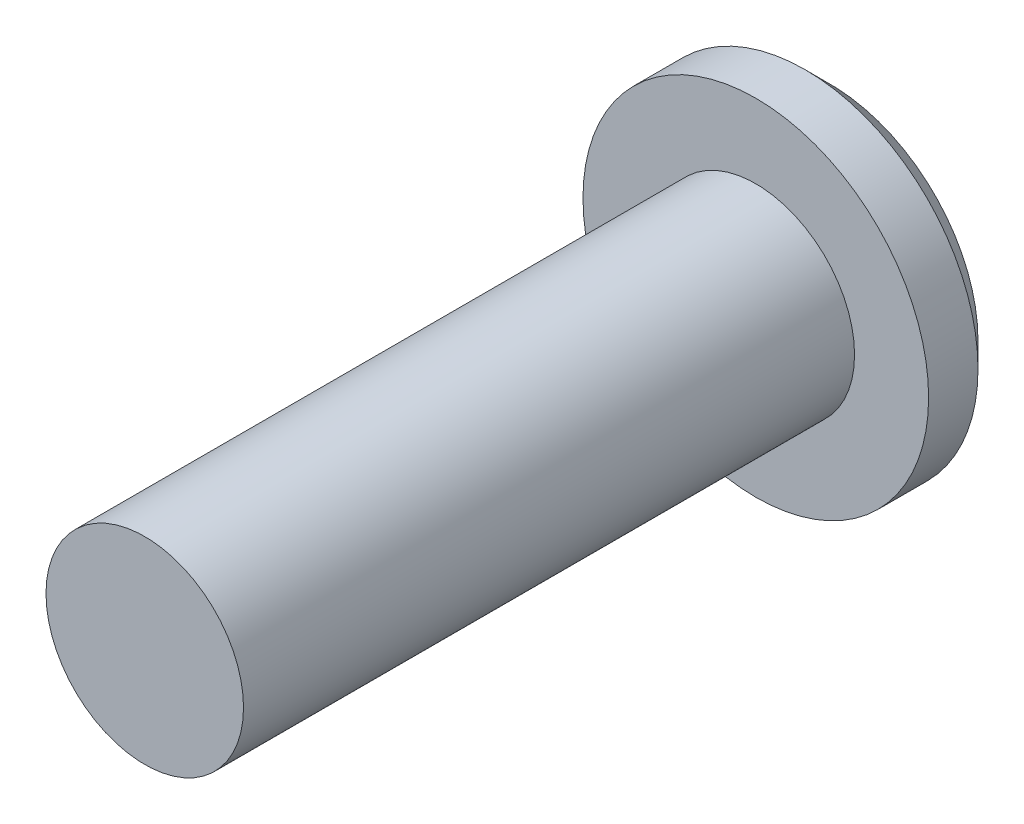
ISO-10303-21;
HEADER;
FILE_DESCRIPTION(('STEP AP214'),'2;1');
FILE_NAME('part.step','',(''),(''),'','','');
FILE_SCHEMA(('AUTOMOTIVE_DESIGN { 1 0 10303 214 1 1 1 1 }'));
ENDSEC;
DATA;
#1=APPLICATION_CONTEXT('core data for automotive mechanical design processes');
#2=APPLICATION_PROTOCOL_DEFINITION('international standard','automotive_design',2000,#1);
#3=PRODUCT_CONTEXT('',#1,'mechanical');
#4=PRODUCT('Part','Part','',(#3));
#5=PRODUCT_RELATED_PRODUCT_CATEGORY('part','',(#4));
#6=PRODUCT_DEFINITION_FORMATION('','',#4);
#7=PRODUCT_DEFINITION_CONTEXT('part definition',#1,'design');
#8=PRODUCT_DEFINITION('design','',#6,#7);
#9=PRODUCT_DEFINITION_SHAPE('','',#8);
#10=(LENGTH_UNIT() NAMED_UNIT(*) SI_UNIT(.MILLI.,.METRE.));
#11=(NAMED_UNIT(*) PLANE_ANGLE_UNIT() SI_UNIT($,.RADIAN.));
#12=(NAMED_UNIT(*) SI_UNIT($,.STERADIAN.) SOLID_ANGLE_UNIT());
#13=UNCERTAINTY_MEASURE_WITH_UNIT(LENGTH_MEASURE(1.E-05),#10,'distance_accuracy_value','');
#14=(GEOMETRIC_REPRESENTATION_CONTEXT(3) GLOBAL_UNCERTAINTY_ASSIGNED_CONTEXT((#13)) GLOBAL_UNIT_ASSIGNED_CONTEXT((#10,
#11,#12)) REPRESENTATION_CONTEXT('',''));
#15=CARTESIAN_POINT('',(0.,0.,0.));
#16=DIRECTION('',(0.,0.,1.));
#17=DIRECTION('',(1.,0.,0.));
#18=AXIS2_PLACEMENT_3D('',#15,#16,#17);
#19=CARTESIAN_POINT('',(0.,0.,3.));
#20=DIRECTION('',(0.,0.,-1.));
#21=DIRECTION('',(-1.,0.,0.));
#22=AXIS2_PLACEMENT_3D('',#19,#20,#21);
#23=CYLINDRICAL_SURFACE('',#22,7.);
#24=CARTESIAN_POINT('',(0.,0.,0.999999999999999));
#25=DIRECTION('',(0.,0.,1.));
#26=DIRECTION('',(1.,0.,0.));
#27=AXIS2_PLACEMENT_3D('',#24,#25,#26);
#28=CIRCLE('',#27,7.);
#29=CARTESIAN_POINT('',(7.,0.,0.999999999999999));
#30=VERTEX_POINT('',#29);
#31=EDGE_CURVE('E52',#30,#30,#28,.T.);
#32=ORIENTED_EDGE('',*,*,#31,.T.);
#33=EDGE_LOOP('',(#32));
#34=FACE_BOUND('',#33,.T.);
#35=CARTESIAN_POINT('',(0.,0.,3.));
#36=DIRECTION('',(0.,0.,1.));
#37=DIRECTION('',(1.,0.,0.));
#38=AXIS2_PLACEMENT_3D('',#35,#36,#37);
#39=CIRCLE('',#38,7.);
#40=CARTESIAN_POINT('',(7.,0.,3.));
#41=VERTEX_POINT('',#40);
#42=EDGE_CURVE('E61',#41,#41,#39,.T.);
#43=ORIENTED_EDGE('',*,*,#42,.F.);
#44=EDGE_LOOP('',(#43));
#45=FACE_BOUND('',#44,.T.);
#46=ADVANCED_FACE('F44',(#34,#45),#23,.T.);
#47=CARTESIAN_POINT('',(0.,0.,3.));
#48=DIRECTION('',(0.,0.,1.));
#49=DIRECTION('',(1.,0.,0.));
#50=AXIS2_PLACEMENT_3D('',#47,#48,#49);
#51=PLANE('',#50);
#52=CARTESIAN_POINT('',(0.,0.,3.));
#53=DIRECTION('',(0.,0.,1.));
#54=DIRECTION('',(1.,0.,0.));
#55=AXIS2_PLACEMENT_3D('',#52,#53,#54);
#56=CIRCLE('',#55,4.);
#57=CARTESIAN_POINT('',(4.,0.,3.));
#58=VERTEX_POINT('',#57);
#59=EDGE_CURVE('E60',#58,#58,#56,.T.);
#60=ORIENTED_EDGE('',*,*,#59,.F.);
#61=EDGE_LOOP('',(#60));
#62=FACE_BOUND('',#61,.T.);
#63=ORIENTED_EDGE('',*,*,#42,.T.);
#64=EDGE_LOOP('',(#63));
#65=FACE_BOUND('',#64,.T.);
#66=ADVANCED_FACE('F78',(#62,#65),#51,.T.);
#67=CARTESIAN_POINT('',(0.,0.,0.));
#68=DIRECTION('',(0.,0.,1.));
#69=DIRECTION('',(1.,0.,0.));
#70=AXIS2_PLACEMENT_3D('',#67,#68,#69);
#71=PLANE('',#70);
#72=CARTESIAN_POINT('',(0.,0.,0.));
#73=DIRECTION('',(0.,0.,1.));
#74=DIRECTION('',(1.,0.,0.));
#75=AXIS2_PLACEMENT_3D('',#72,#73,#74);
#76=CIRCLE('',#75,6.);
#77=CARTESIAN_POINT('',(6.,0.,0.));
#78=VERTEX_POINT('',#77);
#79=EDGE_CURVE('E10',#78,#78,#76,.F.);
#80=ORIENTED_EDGE('',*,*,#79,.T.);
#81=EDGE_LOOP('',(#80));
#82=FACE_BOUND('',#81,.T.);
#83=ADVANCED_FACE('F73',(#82),#71,.F.);
#84=CARTESIAN_POINT('',(0.,0.,27.75));
#85=DIRECTION('',(0.,0.,-1.));
#86=DIRECTION('',(-1.,0.,0.));
#87=AXIS2_PLACEMENT_3D('',#84,#85,#86);
#88=CYLINDRICAL_SURFACE('',#87,4.);
#89=CARTESIAN_POINT('',(0.,0.,27.75));
#90=DIRECTION('',(0.,0.,1.));
#91=DIRECTION('',(1.,0.,0.));
#92=AXIS2_PLACEMENT_3D('',#89,#90,#91);
#93=CIRCLE('',#92,4.);
#94=CARTESIAN_POINT('',(4.,0.,27.75));
#95=VERTEX_POINT('',#94);
#96=EDGE_CURVE('E64',#95,#95,#93,.T.);
#97=ORIENTED_EDGE('',*,*,#96,.F.);
#98=EDGE_LOOP('',(#97));
#99=FACE_BOUND('',#98,.T.);
#100=ORIENTED_EDGE('',*,*,#59,.T.);
#101=EDGE_LOOP('',(#100));
#102=FACE_BOUND('',#101,.T.);
#103=ADVANCED_FACE('F75',(#99,#102),#88,.T.);
#104=CARTESIAN_POINT('',(0.,0.,27.75));
#105=DIRECTION('',(0.,0.,1.));
#106=DIRECTION('',(1.,0.,0.));
#107=AXIS2_PLACEMENT_3D('',#104,#105,#106);
#108=PLANE('',#107);
#109=ORIENTED_EDGE('',*,*,#96,.T.);
#110=EDGE_LOOP('',(#109));
#111=FACE_BOUND('',#110,.T.);
#112=ADVANCED_FACE('F67',(#111),#108,.T.);
#113=CARTESIAN_POINT('',(0.,0.,0.999999999999999));
#114=DIRECTION('',(0.,0.,1.));
#115=DIRECTION('',(1.,0.,0.));
#116=AXIS2_PLACEMENT_3D('',#113,#114,#115);
#117=CONICAL_SURFACE('',#116,7.,0.78539816339745);
#118=ORIENTED_EDGE('',*,*,#79,.F.);
#119=EDGE_LOOP('',(#118));
#120=FACE_BOUND('',#119,.T.);
#121=ORIENTED_EDGE('',*,*,#31,.F.);
#122=EDGE_LOOP('',(#121));
#123=FACE_BOUND('',#122,.T.);
#124=ADVANCED_FACE('F48',(#120,#123),#117,.T.);
#125=CLOSED_SHELL('',(#46,#66,#83,#103,#112,#124));
#126=MANIFOLD_SOLID_BREP('B2',#125);
#127=ADVANCED_BREP_SHAPE_REPRESENTATION('',(#18,#126),#14);
#128=SHAPE_DEFINITION_REPRESENTATION(#9,#127);
ENDSEC;
END-ISO-10303-21;
